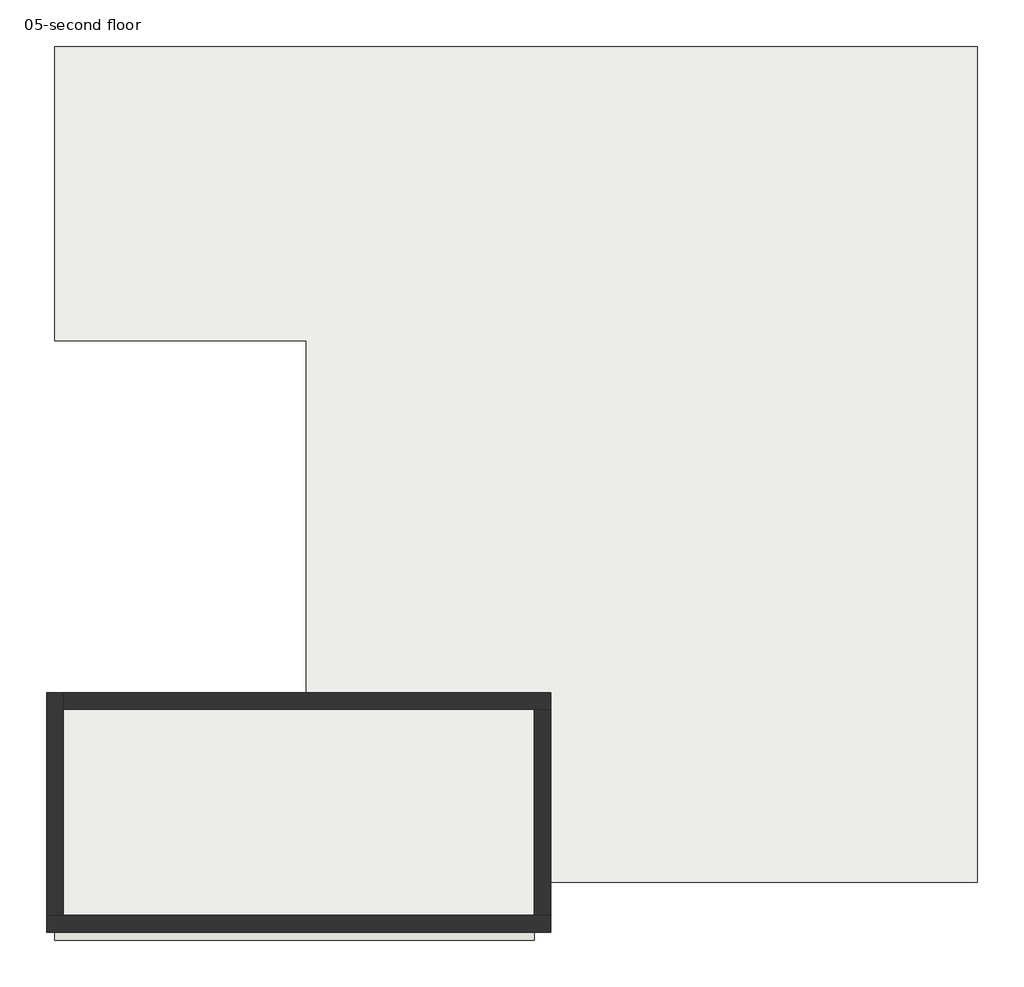
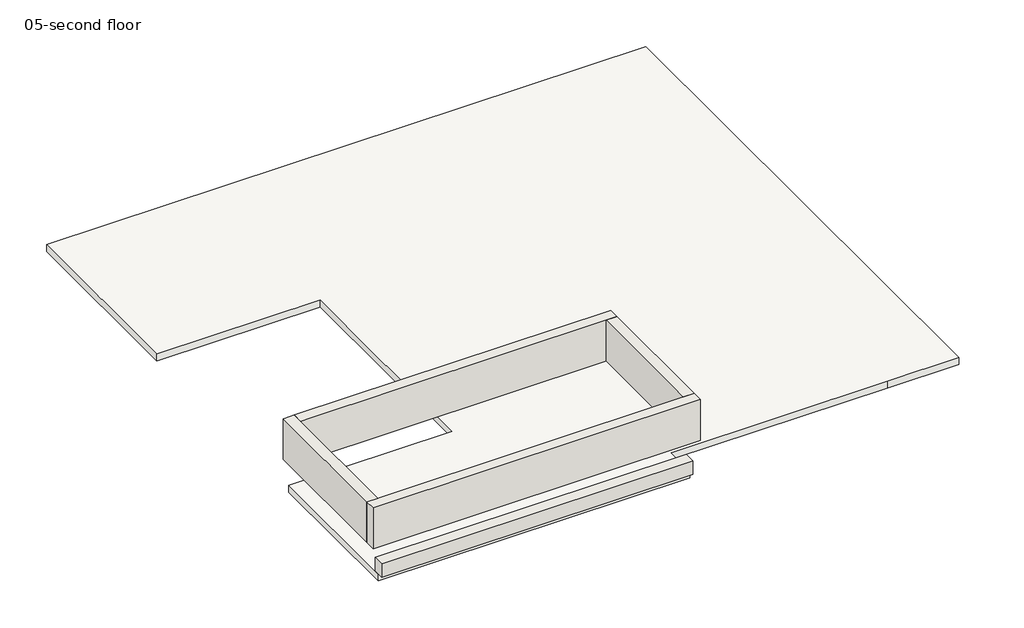
# One storey: 5 walls, 1 slab.
"""IFC4 building model written with IfcOpenShell, lengths in millimetres."""

from ifc_helpers import new_model, si_unit, frame, origin, place, context, project, spatial, polyline, outline, extrude, faceted_brep, element, save

model = new_model("IFC4")

# Units and contexts
model_context = context("Model", 3, world=origin())
ifc_project = project(units=[si_unit("LENGTHUNIT", "METRE", prefix="MILLI")], contexts=[model_context])

# Site, building, storey
site = spatial("IfcSite", under=ifc_project)
building = spatial("IfcBuilding", under=site)
storey = spatial("IfcBuildingStorey", under=building, Name="05-second floor", Elevation=7000.0)

# Slab
placement = place(None, origin())
element("IfcSlab", 1, ObjectType="01-150 floor", at=placement, inside=storey, context=model_context, shape_type="SweptSolid", body=[
    extrude(outline(polyline([(-7995.7520625, 1965.9519156), (-7995.7520625, -9326.0480844), (-9470.7520625, -9326.0480844), (-13987.7520625, -9326.0480844), (-13987.7520625, -10001.0480844), (-20462.7520625, -10001.0480844), (-20462.7520625, -6774.0480844), (-17062.7520625, -6774.0480844), (-17062.7520625, -2009.0480844), (-20462.7520625, -2009.0480844), (-20462.7520625, 1965.9519156), (-7995.7520625, 1965.9519156)])), frame((0.0, 0.0, 6850.0), z_axis=(0.0, 0.0, 1.0), x_axis=(1.0, 0.0, 0.0)), (0.0, 0.0, 1.0), 150.0),
])

# Walls
element("IfcWall", 2, ObjectType="01-225 wall", at=placement, inside=storey, context=model_context, shape_type="SweptSolid", body=[
    extrude(outline(polyline([(-13987.7520625, -10113.5480844), (-20462.7520625, -10113.5480844), (-20462.7520625, -9888.5480844), (-13987.7520625, -9888.5480844), (-13987.7520625, -10113.5480844)])), frame((0.0, 0.0, 7000.0), z_axis=(0.0, 0.0, 1.0), x_axis=(1.0, 0.0, 0.0)), (0.0, 0.0, 1.0), 300.0),
])
element("IfcWall", 3, ObjectType="01-225 wall", at=placement, inside=storey, context=model_context, shape_type="Brep", body=[
    faceted_brep([(-20575.2520625, -10001.0480844, 7600.0), (-13762.7520625, -10001.0480844, 7600.0), (-13762.7520625, -10001.0480844, 8500.0), (-20575.2520625, -10001.0480844, 8500.0), (-20575.2520625, -9776.0480844, 7600.0), (-20575.2520625, -9776.0480844, 8500.0), (-20350.2520625, -9776.0480844, 8500.0), (-13987.7520625, -9776.0480844, 8500.0), (-13762.7520625, -9776.0480844, 8500.0), (-13762.7520625, -9776.0480844, 7600.0), (-13987.7520625, -9776.0480844, 7600.0), (-20350.2520625, -9776.0480844, 7600.0)], [[[0, 1, 2, 3]], [[4, 5, 6, 7, 8, 9, 10, 11]], [[1, 0, 4, 11, 10, 9]], [[3, 2, 8, 7, 6, 5]], [[0, 3, 5, 4]], [[2, 1, 9, 8]]]),
])
element("IfcWall", 4, ObjectType="01-225 wall", at=placement, inside=storey, context=model_context, shape_type="Brep", body=[
    faceted_brep([(-20350.2520625, -9776.0480844, 7600.0), (-20350.2520625, -6988.5480844, 7600.0), (-20350.2520625, -6763.5480844, 7600.0), (-20350.2520625, -6763.5480844, 8500.0), (-20350.2520625, -6988.5480844, 8500.0), (-20350.2520625, -9776.0480844, 8500.0), (-20575.2520625, -9776.0480844, 7600.0), (-20575.2520625, -9776.0480844, 8500.0), (-20575.2520625, -6763.5480844, 8500.0), (-20575.2520625, -6763.5480844, 7600.0)], [[[0, 1, 2, 3, 4, 5]], [[6, 7, 8, 9]], [[2, 1, 0, 6, 9]], [[5, 4, 3, 8, 7]], [[0, 5, 7, 6]], [[3, 2, 9, 8]]]),
])
element("IfcWall", 5, ObjectType="01-225 wall", at=placement, inside=storey, context=model_context, shape_type="Brep", body=[
    faceted_brep([(-20350.2520625, -6988.5480844, 7600.0), (-13987.7520625, -6988.5480844, 7600.0), (-13762.7520625, -6988.5480844, 7600.0), (-13762.7520625, -6988.5480844, 8500.0), (-13987.7520625, -6988.5480844, 8500.0), (-20350.2520625, -6988.5480844, 8500.0), (-20350.2520625, -6763.5480844, 7600.0), (-20350.2520625, -6763.5480844, 8500.0), (-13762.7520625, -6763.5480844, 8500.0), (-13762.7520625, -6763.5480844, 7600.0)], [[[0, 1, 2, 3, 4, 5]], [[6, 7, 8, 9]], [[2, 1, 0, 6, 9]], [[5, 4, 3, 8, 7]], [[0, 5, 7, 6]], [[3, 2, 9, 8]]]),
])
element("IfcWall", 6, ObjectType="01-225 wall", at=placement, inside=storey, context=model_context, shape_type="SweptSolid", body=[
    extrude(outline(polyline([(-13987.7520625, -9776.0480844), (-13987.7520625, -6988.5480844), (-13762.7520625, -6988.5480844), (-13762.7520625, -9776.0480844), (-13987.7520625, -9776.0480844)])), frame((0.0, 0.0, 7600.0), z_axis=(0.0, 0.0, 1.0), x_axis=(1.0, 0.0, 0.0)), (0.0, 0.0, 1.0), 900.0),
])

save(model, "model.ifc")

# Revit data of these elements
# Type "01-150 floor"
#   Description = "Generic Floor (Material By Category), 12\" thick"
#   Assembly Code = "B1010"
#   Type Mark = "G01"
#   Function = 0
#   Layers, outside or top first: 150 mm no material (function 1)
# Type "01-225 wall"
#   Description = "Generic Wall (Material By Category), 200mm thick"
#   Assembly Code = "B2010"
#   Type Mark = "G06"
#   Layers, outside or top first: 225 mm "01-225 main wall" (function 1)
# Element 1 (IfcSlab, "01-150 floor")
#   Height Offset From Level = 0 mm
#   Phase Created = New Construction
#   Materials on its faces: "Default Floor"
# Element 2 (IfcWall, "01-225 wall")
#   Top Offset = 0 mm
#   Base Offset = 0 mm
#   Unconnected Height = 300 mm
#   wall height = 300 mm
#   Phase Created = New Construction
#   Base Constraint = 05-second floor
#   Materials on its faces: "01-225 main wall"
# Elements 3, 4, 5, 6 (IfcWall, "01-225 wall")
#   built-in parameter 1001111 = 600 mm
#   Top Offset = 0 mm
#   Base Offset = 600 mm
#   wall height = 900 mm
#   Phase Created = New Construction
#   Base Constraint = 05-second floor
#   Top Constraint = 04-ceiling-3
#   Materials on its faces: "01-225 main wall"
# Materials
#   "01-225 main wall": class "Generic", colour RGB 244 244 244, transparency 0, Cost = 0
#   "Default Floor": colour RGB 128 128 128, transparency 0, Cost = 0
